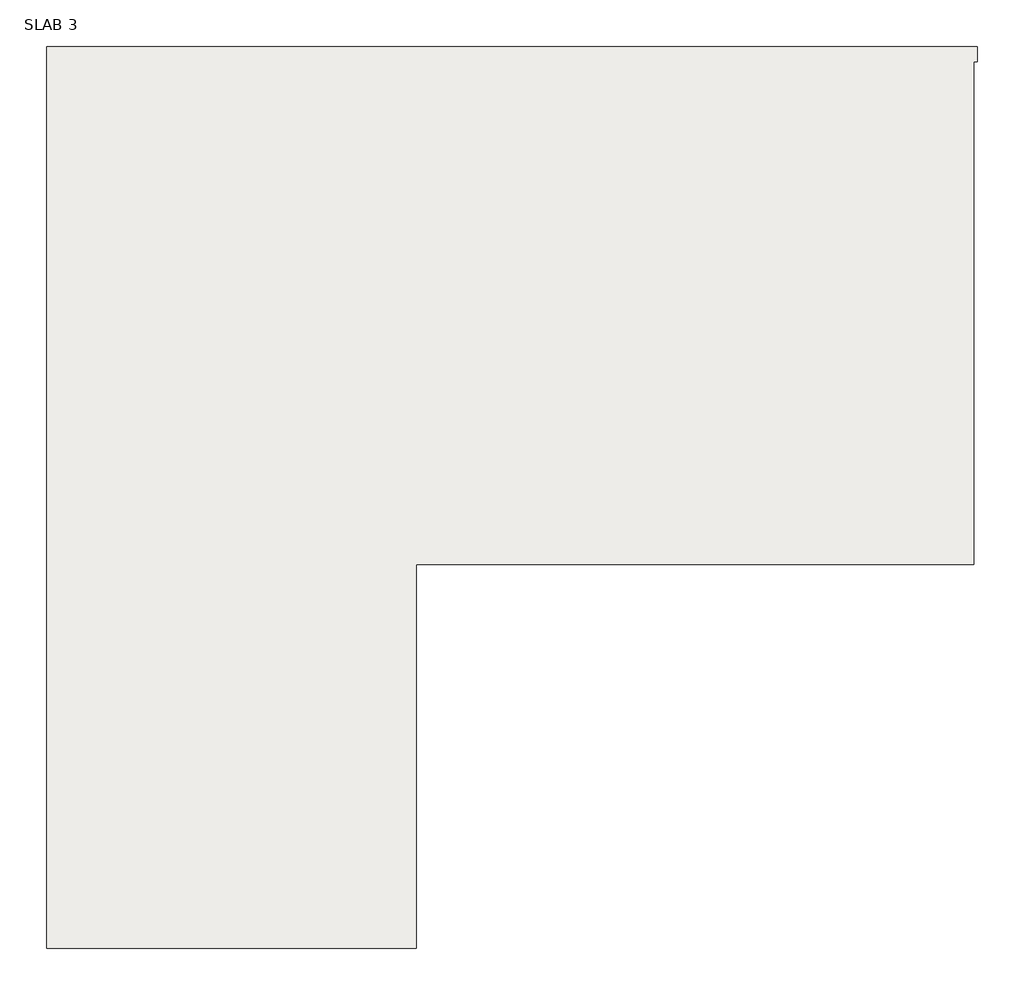
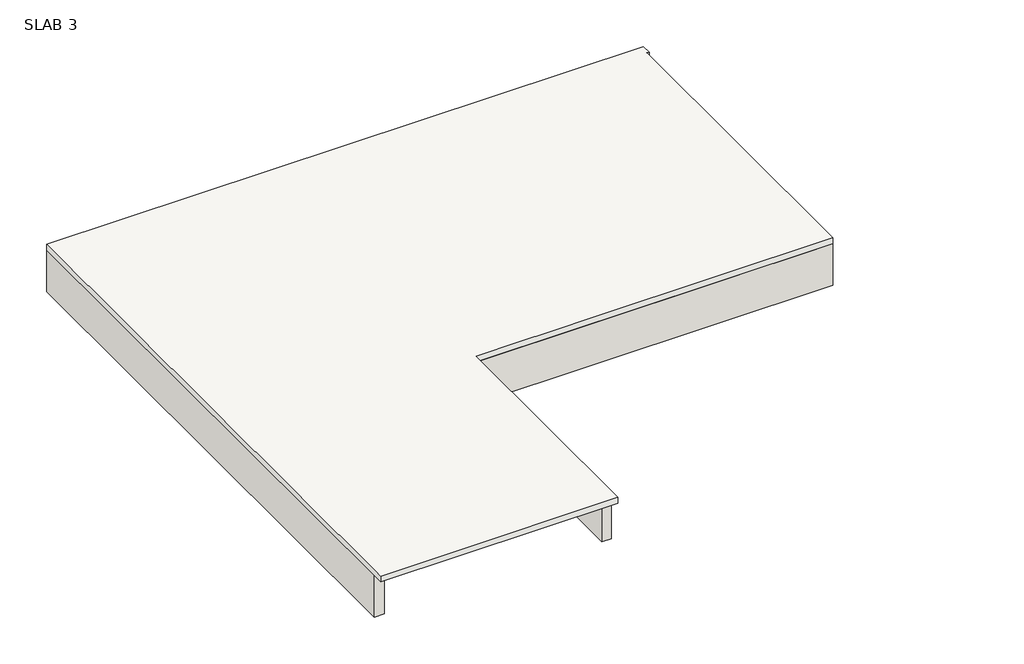
# One storey: 5 walls, 1 roof.
"""IFC4 building model written with IfcOpenShell, lengths in millimetres."""

from ifc_helpers import new_model, si_unit, frame, origin, place, context, project, spatial, polyline, outline, extrude, faceted_brep, element, save

model = new_model("IFC4")

# Units and contexts
model_context = context("Model", 3, world=origin())
ifc_project = project(units=[si_unit("LENGTHUNIT", "METRE", prefix="MILLI")], contexts=[model_context])

# Site, building, storey
site = spatial("IfcSite", under=ifc_project)
building = spatial("IfcBuilding", under=site)
storey = spatial("IfcBuildingStorey", under=building, Name="SLAB 3", Elevation=7924.8)

# Roof
placement = place(None, origin())
element("IfcRoof", 1, ObjectType="Generic - 9\"", at=placement, inside=storey, context=model_context, shape_type="SweptSolid", body=[
    extrude(outline(polyline([(-743.3008651, 13435.9047421), (-743.3008651, 13232.7047421), (-794.1008651, 13232.7047421), (-794.1008651, 6527.1047421), (-8223.6008651, 6527.1047421), (-8223.6008651, 1409.0047421), (-13154.5324866, 1409.0047421), (-13154.5324866, 13435.9047421), (-743.3008651, 13435.9047421)])), frame((0.0, 0.0, 7924.8), z_axis=(0.0, 0.0, 1.0), x_axis=(1.0, 0.0, 0.0)), (0.0, 0.0, 1.0), 127.0),
])

# Walls
element("IfcWall", 2, ObjectType="Generic - 8\"", at=placement, inside=storey, context=model_context, shape_type="Brep", body=[
    faceted_brep([(-8223.6008651, 1637.6047421, 7010.4), (-8223.6008651, 6527.1047421, 7010.4), (-8223.6008651, 6730.3047421, 7010.4), (-8223.6008651, 6730.3047421, 7924.8), (-8223.6008651, 6527.1047421, 7924.8), (-8223.6008651, 1637.6047421, 7924.8), (-8426.8008651, 1637.6047421, 7010.4), (-8426.8008651, 1637.6047421, 7924.8), (-8426.8008651, 6730.3047421, 7924.8), (-8426.8008651, 6730.3047421, 7010.4)], [[[0, 1, 2, 3, 4, 5]], [[6, 7, 8, 9]], [[2, 1, 0, 6, 9]], [[0, 5, 7, 6]], [[3, 2, 9, 8]], [[5, 4, 3, 8, 7]]]),
])
element("IfcWall", 3, ObjectType="Generic - 8\"", at=placement, inside=storey, context=model_context, shape_type="Brep", body=[
    faceted_brep([(-8223.6008651, 6527.1047421, 7010.4), (-794.1008651, 6527.1047421, 7010.4), (-794.1008651, 6527.1047421, 7924.8), (-8223.6008651, 6527.1047421, 7924.8), (-8223.6008651, 6730.3047421, 7010.4), (-8223.6008651, 6730.3047421, 7924.8), (-997.3008651, 6730.3047421, 7924.8), (-794.1008651, 6730.3047421, 7924.8), (-794.1008651, 6730.3047421, 7010.4), (-997.3008651, 6730.3047421, 7010.4)], [[[0, 1, 2, 3]], [[4, 5, 6, 7, 8, 9]], [[1, 0, 4, 9, 8]], [[0, 3, 5, 4]], [[2, 1, 8, 7]], [[3, 2, 7, 6, 5]]]),
])
element("IfcWall", 4, ObjectType="Generic - 8\"", at=placement, inside=storey, context=model_context, shape_type="Brep", body=[
    faceted_brep([(-12948.0008651, 1637.6047421, 7010.4), (-12948.0008651, 13232.7047421, 7010.4), (-12948.0008651, 13435.9047421, 7010.4), (-12948.0008651, 13435.9047421, 7924.8), (-12948.0008651, 13232.7047421, 7924.8), (-12948.0008651, 1637.6047421, 7924.8), (-13151.2008651, 1637.6047421, 7010.4), (-13151.2008651, 1637.6047421, 7924.8), (-13151.2008651, 13435.9047421, 7924.8), (-13151.2008651, 13435.9047421, 7010.4)], [[[0, 1, 2, 3, 4, 5]], [[6, 7, 8, 9]], [[2, 1, 0, 6, 9]], [[0, 5, 7, 6]], [[3, 2, 9, 8]], [[5, 4, 3, 8, 7]]]),
])
element("IfcWall", 5, ObjectType="Generic - 8\"", at=placement, inside=storey, context=model_context, shape_type="Brep", body=[
    faceted_brep([(-12948.0008651, 13232.7047421, 7010.4), (-997.3008651, 13232.7047421, 7010.4), (-794.1008651, 13232.7047421, 7010.4), (-743.3008651, 13232.7047421, 7010.4), (-743.3008651, 13232.7047421, 7924.8), (-794.1008651, 13232.7047421, 7924.8), (-997.3008651, 13232.7047421, 7924.8), (-12948.0008651, 13232.7047421, 7924.8), (-12948.0008651, 13435.9047421, 7010.4), (-12948.0008651, 13435.9047421, 7924.8), (-743.3008651, 13435.9047421, 7924.8), (-743.3008651, 13435.9047421, 7010.4)], [[[0, 1, 2, 3, 4, 5, 6, 7]], [[8, 9, 10, 11]], [[3, 2, 1, 0, 8, 11]], [[4, 3, 11, 10]], [[0, 7, 9, 8]], [[7, 6, 5, 4, 10, 9]]]),
])
element("IfcWall", 6, ObjectType="Generic - 8\"", at=placement, inside=storey, context=model_context, shape_type="SweptSolid", body=[
    extrude(outline(polyline([(-997.3008651, 6730.3047421), (-997.3008651, 13232.7047421), (-794.1008651, 13232.7047421), (-794.1008651, 6730.3047421), (-997.3008651, 6730.3047421)])), frame((0.0, 0.0, 7010.4), z_axis=(0.0, 0.0, 1.0), x_axis=(1.0, 0.0, 0.0)), (0.0, 0.0, 1.0), 914.4),
])

save(model, "model.ifc")

# Revit data of these elements
# Type "Generic - 9\""
#   Assembly Code = "B1020"
#   Layers, outside or top first: 0' - 5" "WHITE" (function 1)
# Type "Generic - 8\""
#   Assembly Code = "B2010"
#   Layers, outside or top first: 0' - 8" "Default New Material(1)" (function 1)
# Element 1 (IfcRoof, "Generic - 9\"")
#   built-in parameter 1001705 = 26.4167 (stored number, unit not read)
#   built-in parameter 1001710 = 33615
#   Phase Created = New Construction
#   Materials on its faces: "WHITE"
# Elements 2, 3, 4, 5, 6 (IfcWall, "Generic - 8\"")
#   built-in parameter 1001111 = -3' - 0"
#   Top Offset = 0' - 0"
#   Base Offset = -3' - 0"
#   Unconnected Height = 5' - 0"
#   wall height = 5' - 0"
#   Phase Created = New Construction
#   Base Constraint = SLAB 3
#   Materials on its faces: "Default New Material(1)"
# Materials
#   "WHITE": class "Generic", colour RGB 255 255 255, transparency 0, Cost = 0
#   "Default New Material(1)": class "Generic", colour RGB 192 192 192, transparency 0, Cost = 0
